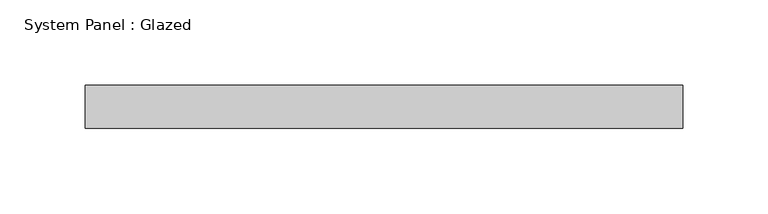
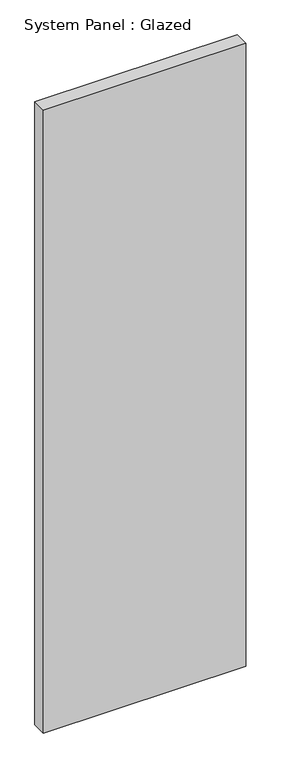
"""IFC4 building model written with IfcOpenShell, lengths in millimetres: plate geometry, System Panel : Glazed."""

from ifc_helpers import new_model, si_unit, origin, origin_with_axes, place, context, project, spatial, polyline, outline, extrude, source, transform, mapped, element, save


def system_panel_glazed_6a35409e(model_context):
    return source(origin(), model_context, "Body", "SweptSolid", [
        extrude(outline(polyline([(175.6833333, 19.05), (-175.6833333, 19.05), (-175.6833333, 44.45), (175.6833333, 44.45), (175.6833333, 19.05)])), origin_with_axes(), (0.0, 0.0, 1.0), 1143.0),
    ])


if __name__ == "__main__":
    model = new_model("IFC4")
    model_context = context("Model", 3, world=origin())
    ifc_project = project(units=[si_unit("LENGTHUNIT", "METRE", prefix="MILLI")], contexts=[model_context])
    site = spatial("IfcSite", under=ifc_project)
    building = spatial("IfcBuilding", under=site)
    placement = place(None, origin())
    system_panel_glazed_shape = system_panel_glazed_6a35409e(model_context)
    element("IfcPlate", 1, ObjectType="System Panel : Glazed", at=placement, inside=building, context=model_context, shape_type="MappedRepresentation", body=[
        mapped(system_panel_glazed_shape, transform((0.0, 0.0, 0.0), x_axis=(1.0, 0.0, 0.0), y_axis=(0.0, 1.0, 0.0), z_axis=(0.0, 0.0, 1.0))),
    ])
    save(model, "model.ifc")

# Revit data of these elements
# Type "System Panel : Glazed"
#   Construction Type Id = "GSP4R"
#   Analytic Construction = "1/8 in Pilkington single glazing"
#   Visual Light Transmittance = 0.9
#   Solar Heat Gain Coefficient = 0.86
#   Heat Transfer Coefficient (U) = 1.18115 BTU/(h·ft²·°F)
#   Define Thermal Properties by = 1
# Element 1 (IfcPlate, "System Panel : Glazed")
#   Materials on its faces: "Glass"
# Materials
#   "Glass": class "Glass", colour RGB 0 128 192, transparency 0.75, Description = "Soda Lime Glass", Cost = 0
